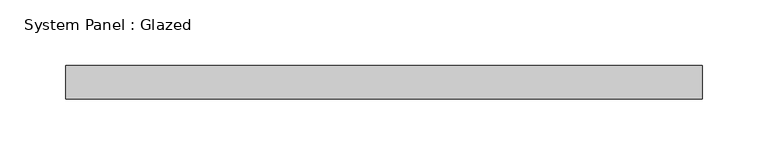
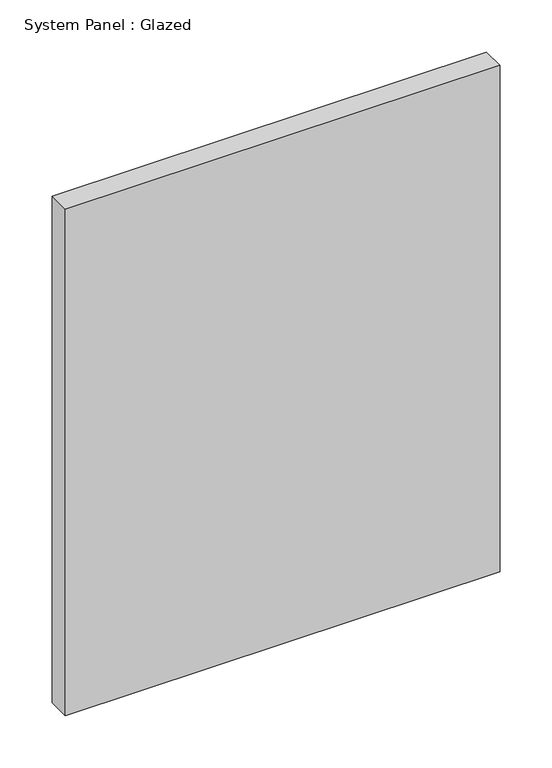
"""IFC4 building model written with IfcOpenShell, lengths in millimetres: plate geometry, System Panel : Glazed."""

from ifc_helpers import new_model, si_unit, origin, origin_with_axes, place, context, project, spatial, polyline, outline, extrude, source, transform, mapped, element, save


def system_panel_glazed_625789f6(model_context):
    return source(origin(), model_context, "Body", "SweptSolid", [
        extrude(outline(polyline([(241.3, 19.05), (-241.3, 19.05), (-241.3, 44.45), (241.3, 44.45), (241.3, 19.05)])), origin_with_axes(), (0.0, 0.0, 1.0), 594.5951495),
    ])


if __name__ == "__main__":
    model = new_model("IFC4")
    model_context = context("Model", 3, world=origin())
    ifc_project = project(units=[si_unit("LENGTHUNIT", "METRE", prefix="MILLI")], contexts=[model_context])
    site = spatial("IfcSite", under=ifc_project)
    building = spatial("IfcBuilding", under=site)
    placement = place(None, origin())
    system_panel_glazed_shape = system_panel_glazed_625789f6(model_context)
    element("IfcPlate", 1, ObjectType="System Panel : Glazed", at=placement, inside=building, context=model_context, shape_type="MappedRepresentation", body=[
        mapped(system_panel_glazed_shape, transform((0.0, 0.0, 0.0), x_axis=(1.0, 0.0, 0.0), y_axis=(0.0, 1.0, 0.0), z_axis=(0.0, 0.0, 1.0))),
    ])
    save(model, "model.ifc")

# Revit data of these elements
# Type "System Panel : Glazed"
#   Construction Type Id = "GSP4R"
#   Analytic Construction = "1/8 in Pilkington single glazing"
#   Visual Light Transmittance = 0.9
#   Solar Heat Gain Coefficient = 0.86
#   Heat Transfer Coefficient (U) = 1.18115 BTU/(h·ft²·°F)
#   Define Thermal Properties by = 1
# Element 1 (IfcPlate, "System Panel : Glazed")
#   Materials on its faces: "Glass"
# Materials
#   "Glass": class "Glass", colour RGB 0 128 192, transparency 0.75, Description = "Soda Lime Glass", Cost = 0
